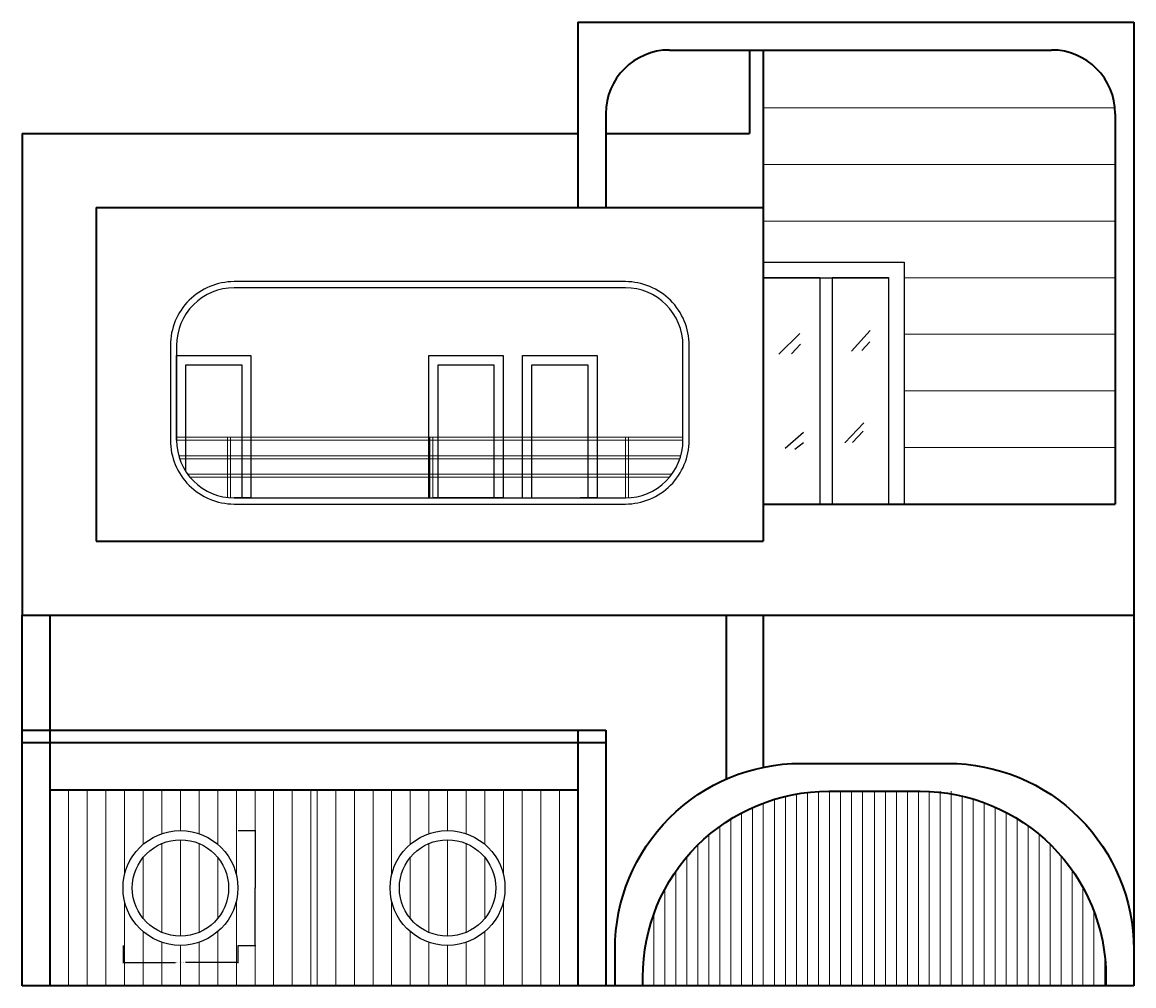
# Model space of a CAD drawing. Units: inches. Extents: x 183 to 543, y 128 to 440.
import ezdxf

# ---------------------------------------------------------------- set-up
doc = ezdxf.new("R2010")
doc.units = ezdxf.units.IN
doc.header["$MEASUREMENT"] = 0
for name, color, linetype, lineweight in [('A-ANNO-DIMS', 2, 'Continuous', 18), ('A-DOOR', 4, 'Continuous', 25), ('A-ELEV', 7, 'Continuous', 35), ('A-ELEV-PATT', 8, 'Continuous', 13), ('A-ELEV-RAIL', 6, 'Continuous', 18), ('A-GLAZ', 3, 'Continuous', 25)]:
    doc.layers.add(name, color=color, linetype=linetype, lineweight=lineweight)
doc.styles.get("Standard").update_dxf_attribs({"font": 'arial.ttf'})
doc.dimstyles.get("Standard").update_dxf_attribs({"dimtxt": 0.18, "dimasz": 0.18, "dimexe": 0.18, "dimexo": 0.0625, "dimgap": 0.09, "dimtad": 0, "dimtih": 1, "dimtoh": 1, "dimdec": 4, "dimzin": 0, "dimdsep": 46, "dimtxsty": 'Standard', "dimcen": 0.09, "dimadec": 0, "dimazin": 0, "dimtfac": 1, "dimtdec": 4, "dimtofl": 0, "dimtmove": 0, "dimatfit": 3, "dimfxl": 1, "dimtolj": 1, "dimtzin": 0, "dimarcsym": 0})

# ---------------------------------------------------------------- blocks, each defined once
blk = doc.blocks.new('WIN-ROUND')
for radius in [18.6, 15.6]:
    blk.add_circle((234.26, 159.86), radius)
blk = doc.blocks.new('*D2')
at = {"layer": 'A-ANNO-DIMS', "color": 0, "lineweight": -2, "transparency": 16777216}
for p, q in [((215.67, 141.2), (215.67, 135.5)), ((252.86, 141.2), (252.86, 135.5)), ((215.85, 135.68), (232.66, 135.68)), ((252.68, 135.68), (235.87, 135.68))]:
    blk.add_line(p, q, dxfattribs=at)
at = {"layer": 'A-ANNO-DIMS', "color": 0, "transparency": 16777216}
for points in [[(215.85, 135.71), (215.85, 135.65), (215.67, 135.68)], [(252.68, 135.71), (252.68, 135.65), (252.86, 135.68)]]:
    blk.add_solid(points, dxfattribs=at)
at = {"layer": 'Defpoints', "color": 0, "transparency": 16777216}
for p in [(215.67, 141.26), (252.86, 141.26), (252.86, 135.68)]:
    blk.add_point(p, dxfattribs=at)
at = {"layer": 'A-ANNO-DIMS', "color": 0, "transparency": 16777216, "insert": (234.26, 135.68), "char_height": 0.18, "attachment_point": 5}
blk.add_mtext('\\A1;ROUND WINDOW 37 TYP.', dxfattribs=at)
blk = doc.blocks.new('*D3')
at = {"layer": 'A-ANNO-DIMS', "color": 0, "lineweight": -2, "transparency": 16777216}
for p, q in [((252.93, 178.46), (258.62, 178.46)), ((258.44, 178.28), (258.44, 160.04)), ((258.44, 141.44), (258.44, 159.68)), ((252.93, 141.26), (258.62, 141.26))]:
    blk.add_line(p, q, dxfattribs=at)
at = {"layer": 'A-ANNO-DIMS', "color": 0, "transparency": 16777216}
for points in [[(258.41, 178.28), (258.47, 178.28), (258.44, 178.46)], [(258.41, 141.44), (258.47, 141.44), (258.44, 141.26)]]:
    blk.add_solid(points, dxfattribs=at)
at = {"layer": 'Defpoints', "color": 0, "transparency": 16777216}
for p in [(252.86, 178.46), (258.44, 178.46), (252.86, 141.26)]:
    blk.add_point(p, dxfattribs=at)
at = {"layer": 'A-ANNO-DIMS', "color": 0, "transparency": 16777216, "insert": (258.44, 159.86), "char_height": 0.18, "attachment_point": 5}
blk.add_mtext('\\A1;37 TYP.', dxfattribs=at)

msp = doc.modelspace()

# ---------------------------------------------------------------- linework, layer by layer
at = {"layer": 'A-DOOR'}
for p, q in [((422.96, 357.47), (463.63, 357.47)), ((441.32, 357.54), (441.32, 284.19)), ((445.32, 357.54), (445.32, 284.19)), ((428.1, 332.7), (434.88, 339.36)), ((451.55, 333.7), (457.66, 340.36)), ((432.21, 332.81), (435.1, 335.92)), ((454.99, 333.92), (457.55, 336.7)), ((449.43, 304.04), (455.54, 310.48)), ((430.11, 302.27), (436, 307.48)), ((451.88, 304.15), (455.32, 307.82)), ((433.22, 301.94), (436, 304.15))]:
    msp.add_line(p, q, dxfattribs=at)
for points in [[(423.01, 362.54), (468.63, 362.54), (468.63, 284.19)], [(445.32, 357.54), (463.63, 357.54), (463.63, 284.19), (423.01, 284.19), (423.01, 357.54), (441.32, 357.54)], [(233.01, 304.83), (233.01, 332.23), (257.09, 332.23), (257.09, 286.19), (251.65, 286.19)], [(314.68, 286.19), (314.68, 332.23), (338.76, 332.23), (338.76, 286.19), (316.01, 286.19)], [(345.09, 286.19), (345.09, 332.23), (369.17, 332.23), (369.17, 286.19), (363.73, 286.19)], [(236.01, 294.69), (236.01, 329.23), (254.09, 329.23), (254.09, 286.19)], [(317.68, 286.19), (317.68, 329.23), (335.76, 329.23), (335.76, 286.19)], [(348.09, 286.19), (348.09, 329.23), (366.17, 329.23), (366.17, 286.19)]]:
    msp.add_lwpolyline(points, dxfattribs=at)
at = {"layer": 'A-ELEV'}
for p, q in [((363.01, 440.19), (543.01, 440.19)), ((363.01, 440.19), (363.01, 380.19)), ((543.01, 440.19), (543.01, 248.19)), ((392.65, 431.19), (516.38, 431.19)), ((418.57, 431.19), (418.57, 404.19)), ((423.01, 431.19), (423.01, 272.19)), ((372.01, 410.56), (372.01, 380.19)), ((537.01, 410.56), (537.01, 284.19)), ((183.01, 404.19), (363.01, 404.19)), ((183.01, 404.19), (183.01, 248.19)), ((372.01, 404.19), (418.57, 404.19)), ((207.01, 380.19), (423.01, 380.19)), ((207.01, 380.19), (207.01, 272.19)), ((423.01, 284.19), (537.01, 284.19)), ((207.01, 272.19), (423.01, 272.19)), ((183.01, 248.19), (543.01, 248.19)), ((183.01, 128.19), (183.01, 248.19)), ((192.01, 128.19), (192.01, 248.19)), ((411.01, 248.19), (411.01, 195.12)), ((423.01, 248.19), (423.01, 198.94)), ((543.01, 248.19), (543.01, 128.19)), ((183.01, 210.94), (372.01, 210.94)), ((192.01, 128.19), (192.01, 210.94)), ((363.01, 210.94), (363.01, 128.19)), ((372.01, 210.94), (372.01, 128.19)), ((183.01, 206.94), (372.01, 206.94)), ((363.01, 191.53), (192.01, 191.53)), ((543.01, 128.19), (183.01, 128.19)), ((372.01, 128.19), (192.01, 128.19)), ((543.01, 128.19), (375.01, 128.19))]:
    msp.add_line(p, q, dxfattribs=at)
for points in [[(375.01, 128.19), (375.01, 140, -0.414214), (435.21, 200.19), (482.82, 200.19, -0.414214), (543.01, 140), (543.01, 128.19)], [(384.01, 128.19), (384.01, 131, -0.414214), (444.21, 191.19), (473.82, 191.19, -0.414214), (534.01, 131), (534.01, 128.19)]]:
    msp.add_lwpolyline(points, format="xyb", dxfattribs=at)
for centre, start, end in [((392.65, 410.56), 90, 180), ((516.38, 410.56), 0, 90)]:
    msp.add_arc(centre, 20.64, start, end, dxfattribs=at)
at = {"layer": 'A-ELEV-PATT'}
for p, q in [((422.93, 412.43), (536.93, 412.43)), ((422.94, 394.11), (536.94, 394.11)), ((422.95, 375.79), (536.95, 375.79)), ((468.63, 357.47), (536.96, 357.47)), ((468.63, 339.15), (536.98, 339.15)), ((468.63, 320.83), (536.99, 320.83)), ((468.63, 302.51), (537, 302.51)), ((198.05, 191.53), (198.05, 128.19)), ((204.09, 191.53), (204.09, 128.19)), ((210.12, 191.53), (210.12, 128.19)), ((216.16, 191.53), (216.16, 164.1)), ((222.19, 191.53), (222.19, 174.01)), ((228.23, 191.53), (228.23, 177.45)), ((234.26, 191.53), (234.26, 178.46)), ((240.3, 191.53), (240.3, 177.45)), ((246.34, 191.53), (246.34, 174.01)), ((252.37, 191.53), (252.37, 164.1)), ((258.41, 191.53), (258.41, 128.19)), ((264.44, 191.53), (264.44, 128.19)), ((270.48, 191.53), (270.48, 128.19)), ((276.51, 191.53), (276.51, 128.19)), ((278.51, 191.53), (278.51, 128.19)), ((284.55, 191.53), (284.55, 128.19)), ((290.58, 191.53), (290.58, 128.19)), ((296.62, 191.53), (296.62, 128.19)), ((302.65, 191.53), (302.65, 164.1)), ((308.69, 191.53), (308.69, 174.01)), ((314.73, 191.53), (314.73, 177.45)), ((320.76, 191.53), (320.76, 178.46)), ((326.8, 191.53), (326.8, 177.45)), ((332.83, 191.53), (332.83, 174.01)), ((338.87, 191.53), (338.87, 164.1)), ((344.91, 191.53), (344.91, 128.19)), ((350.94, 191.53), (350.94, 128.19)), ((356.98, 191.53), (356.98, 128.19)), ((363.01, 191.53), (363.01, 128.19)), ((440.9, 191.19), (440.9, 128.19)), ((444.46, 191.19), (444.46, 128.19)), ((448.01, 191.19), (448.01, 128.19)), ((451.57, 191.19), (451.57, 128.19)), ((455.12, 191.19), (455.12, 128.19)), ((459.01, 191.19), (459.01, 128.19)), ((462.57, 191.19), (462.57, 128.19)), ((466.12, 191.19), (466.12, 128.19)), ((469.68, 191.19), (469.68, 128.19)), ((473.24, 191.19), (473.24, 128.19)), ((476.79, 191.19), (476.79, 128.19)), ((480.35, 191.19), (480.35, 128.19)), ((483.9, 191.19), (483.9, 128.19)), ((423.01, 187.34), (423.01, 128.19)), ((426.68, 188.58), (426.68, 128.19)), ((430.24, 189.55), (430.24, 128.19)), ((433.79, 190.28), (433.79, 128.19)), ((437.35, 190.8), (437.35, 128.19)), ((487.46, 189.63), (487.46, 128.19)), ((491.01, 188.68), (491.01, 128.19)), ((494.57, 187.5), (494.57, 128.19)), ((416.01, 184.18), (416.01, 128.19)), ((419.57, 185.92), (419.57, 128.19)), ((498.12, 186.07), (498.12, 128.19)), ((501.68, 184.36), (501.68, 128.19)), ((412.46, 182.14), (412.46, 128.19)), ((505.24, 182.34), (505.24, 128.19)), ((405.35, 176.97), (405.35, 128.19)), ((408.9, 179.75), (408.9, 128.19)), ((508.79, 179.99), (508.79, 128.19)), ((512.35, 177.25), (512.35, 128.19)), ((228.23, 174.24), (228.23, 145.48)), ((234.26, 175.46), (234.26, 144.26)), ((240.3, 174.24), (240.3, 145.48)), ((314.73, 174.24), (314.73, 145.48)), ((320.76, 175.46), (320.76, 144.26)), ((326.8, 174.24), (326.8, 145.48)), ((401.79, 173.71), (401.79, 128.19)), ((515.9, 174.04), (515.9, 128.19)), ((222.19, 169.74), (222.19, 149.98)), ((246.34, 169.74), (246.34, 149.98)), ((308.69, 169.74), (308.69, 149.98)), ((332.83, 169.74), (332.83, 149.98)), ((398.24, 169.85), (398.24, 128.19)), ((519.46, 170.25), (519.46, 128.19)), ((523.01, 165.68), (523.01, 128.19)), ((394.68, 165.21), (394.68, 128.19)), ((391.12, 159.38), (391.12, 128.19)), ((526.57, 159.99), (526.57, 128.19)), ((216.16, 155.62), (216.16, 128.19)), ((252.37, 155.62), (252.37, 128.19)), ((302.65, 155.62), (302.65, 128.19)), ((338.87, 155.62), (338.87, 128.19)), ((387.57, 151.38), (387.57, 128.19)), ((530.12, 152.28), (530.12, 128.19)), ((222.19, 145.71), (222.19, 128.19)), ((246.34, 145.71), (246.34, 128.19)), ((308.69, 145.71), (308.69, 128.19)), ((332.83, 145.71), (332.83, 128.19)), ((228.23, 142.27), (228.23, 128.19)), ((234.26, 141.26), (234.26, 128.19)), ((240.3, 142.27), (240.3, 128.19)), ((314.73, 142.27), (314.73, 128.19)), ((320.76, 141.26), (320.76, 128.19)), ((326.8, 142.27), (326.8, 128.19)), ((533.68, 137.32), (533.68, 128.19)), ((384.01, 131), (384.01, 128.19))]:
    msp.add_line(p, q, dxfattribs=at)
at = {"layer": 'A-ELEV-RAIL'}
for p, q in [((233.01, 305.83), (397.01, 305.83)), ((233.01, 304.83), (397.01, 304.83)), ((249.5, 305.95), (249.5, 286.32)), ((250.5, 305.95), (250.5, 286.32)), ((315.01, 305.83), (315.01, 286.19)), ((316.01, 305.83), (316.01, 286.19)), ((378.38, 305.83), (378.38, 286.19)), ((379.38, 305.83), (379.38, 286.19)), ((233.7, 299.83), (396.33, 299.83)), ((234.01, 298.83), (396.02, 298.83)), ((236.61, 293.83), (393.42, 293.83)), ((237.39, 292.83), (392.64, 292.83))]:
    msp.add_line(p, q, dxfattribs=at)
at = {"layer": 'A-GLAZ'}
for points in [[(399.01, 335.56, 0.414214), (378.38, 356.19), (251.65, 356.19, 0.414214), (231.01, 335.56), (231.01, 304.83, 0.414214), (251.65, 284.19), (378.38, 284.19, 0.414214), (399.01, 304.83)], [(397.01, 335.56, 0.414214), (378.38, 354.19), (251.65, 354.19, 0.414214), (233.01, 335.56), (233.01, 304.83, 0.414214), (251.65, 286.19), (378.38, 286.19, 0.414214), (397.01, 304.83)]]:
    msp.add_lwpolyline(points, format="xyb", close=True, dxfattribs=at)

# ---------------------------------------------------------------- block references
for p in [(0, 0), (86.5, 0)]:
    msp.add_blockref('WIN-ROUND', p, dxfattribs=at)

# ---------------------------------------------------------------- dimensions: what is measured, and where the dimension line sits
at = {"layer": 'A-ANNO-DIMS'}
dim = msp.add_linear_dim(base=(258.44, 178.46), p1=(252.86, 141.26), p2=(252.86, 178.46), angle=90, text='<> TYP.', dimstyle='Standard', override={"dimdec": 0, "dimlfac": 1, "dimrnd": 0, "dimzin": 0, "dimdsep": 46, "dimlunit": 2}, dxfattribs=at)
dim.commit()
dim.dimension.update_dxf_attribs({"geometry": '*D3', "text_midpoint": (258.44, 159.86)})
dim = msp.add_linear_dim(base=(252.86, 135.68), p1=(215.67, 141.26), p2=(252.86, 141.26), text='ROUND WINDOW <> TYP.', dimstyle='Standard', override={"dimdec": 0, "dimlfac": 1, "dimrnd": 0, "dimzin": 0, "dimdsep": 46, "dimlunit": 2}, dxfattribs=at)
dim.commit()
dim.dimension.update_dxf_attribs({"geometry": '*D2', "text_midpoint": (234.26, 135.68)})

doc.saveas('drawing.dxf')
